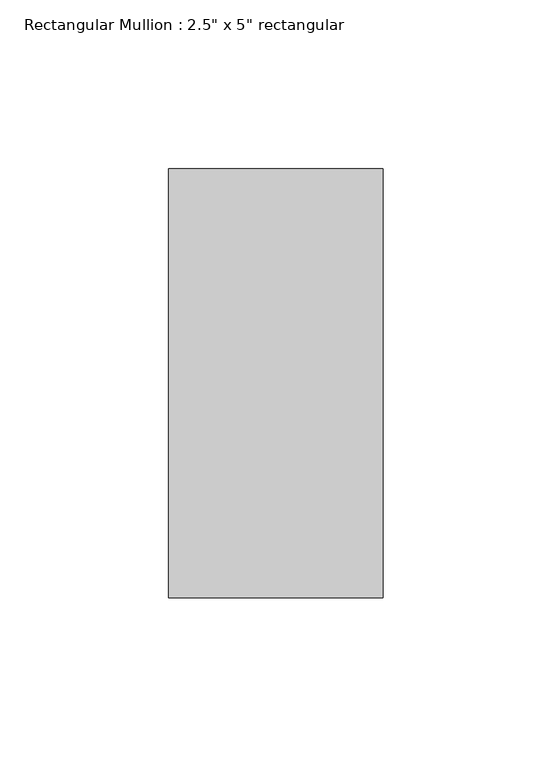
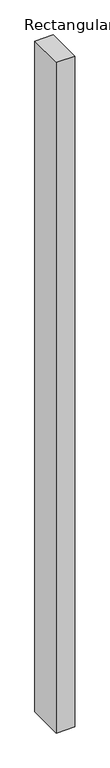
"""IFC4 building model written with IfcOpenShell, lengths in millimetres: member geometry."""

from ifc_helpers import new_model, si_unit, frame, origin, place, context, project, spatial, polyline, outline, extrude, source, transform, mapped, element, save


def member_8e6e9988(model_context):
    return source(origin(), model_context, "Body", "SweptSolid", [
        extrude(outline(polyline([(31.75, 63.5), (31.75, -63.5), (-31.75, -63.5), (-31.75, 63.5), (31.75, 63.5)])), frame((0.0, 0.0, -2444.75), z_axis=(0.0, 0.0, 1.0), x_axis=(1.0, 0.0, 0.0)), (0.0, 0.0, 1.0), 2444.75),
    ])


if __name__ == "__main__":
    model = new_model("IFC4")
    model_context = context("Model", 3, world=origin())
    ifc_project = project(units=[si_unit("LENGTHUNIT", "METRE", prefix="MILLI")], contexts=[model_context])
    site = spatial("IfcSite", under=ifc_project)
    building = spatial("IfcBuilding", under=site)
    placement = place(None, origin())
    member_shape = member_8e6e9988(model_context)
    element("IfcMember", 1, ObjectType="Rectangular Mullion : 2.5\" x 5\" rectangular", at=placement, inside=building, context=model_context, shape_type="MappedRepresentation", body=[
        mapped(member_shape, transform((0.0, 0.0, 0.0), x_axis=(1.0, 0.0, 0.0), y_axis=(0.0, 1.0, 0.0), z_axis=(0.0, 0.0, 1.0))),
    ])
    save(model, "model.ifc")

# Revit data of these elements
# Type "Rectangular Mullion : 2.5\" x 5\" rectangular"
#   built-in parameter 1007304 = 0.416667 (stored number, unit not read)
#   built-in parameter 1007301 = 0.104167 (stored number, unit not read)
#   built-in parameter 1007300 = 0.104167 (stored number, unit not read)
# Element 1 (IfcMember, "Rectangular Mullion : 2.5\" x 5\" rectangular")
#   Materials on its faces: "Aluminum"
# Materials
#   "Aluminum": class "Metal", colour RGB 247 247 247, transparency 0, Description = "Aluminum 6061", Cost = 0
